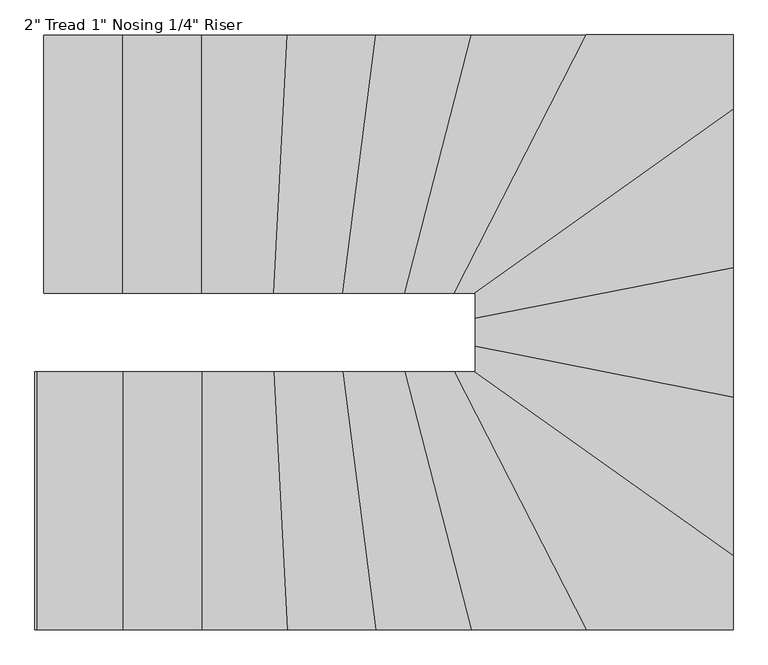
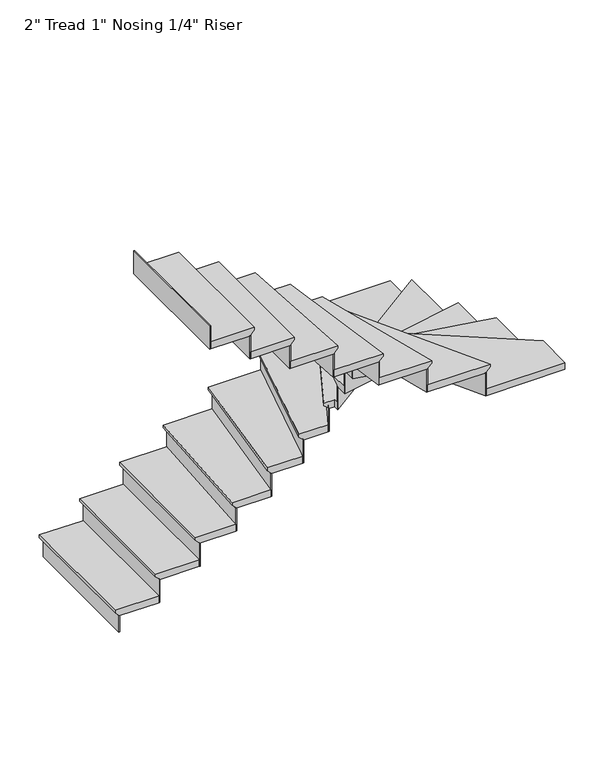
"""IFC4 building model written with IfcOpenShell, lengths in millimetres: stair flight geometry."""

from ifc_helpers import new_model, si_unit, origin, place, context, project, spatial, faceted_brep, source, transform, mapped, element, save


def stair_flight_469f198f(model_context):
    return source(origin(), model_context, "Body", "Brep", [
        faceted_brep([(-3203.9558053, -1112.1366944, 150.2833333), (-3203.9558053, -1112.1366944, 169.3333333), (-3203.9558053, -197.7366944, 169.3333333), (-3203.9558053, -197.7366944, 150.2833333), (-3178.5558053, -1112.1366944, 124.8833333), (-3178.5558053, -197.7366944, 124.8833333), (-2899.1558053, -1112.1366944, 169.3333333), (-2899.1558053, -197.7366944, 169.3333333), (-3178.5558053, -197.7366944, 118.5333333), (-2899.1558053, -197.7366944, 118.5333333), (-2899.1558053, -1112.1366944, 118.5333333), (-3178.5558053, -1112.1366944, 118.5333333)], [[[0, 1, 2, 3]], [[4, 0, 3, 5]], [[2, 1, 6, 7]], [[8, 9, 10, 11]], [[2, 7, 9, 8, 5, 3]], [[8, 11, 4, 5]], [[6, 1, 0, 4, 11, 10]], [[7, 6, 10, 9]]]),
        faceted_brep([(-3178.5558053, -1112.1366944, 118.5333333), (-3178.5558053, -1112.1366944, 0.0), (-3172.2058053, -1112.1366944, 0.0), (-3172.2058053, -1112.1366944, 118.5333333), (-3178.5558053, -197.7366944, 118.5333333), (-3172.2058053, -197.7366944, 118.5333333), (-3172.2058053, -197.7366944, 0.0), (-3178.5558053, -197.7366944, 0.0)], [[[0, 1, 2, 3]], [[4, 5, 6, 7]], [[1, 0, 4, 7]], [[2, 1, 7, 6]], [[3, 2, 6, 5]], [[0, 3, 5, 4]]]),
        faceted_brep([(-2899.1558053, -1112.1366944, 287.8666667), (-2899.1558053, -1112.1366944, 118.5333333), (-2892.8058053, -1112.1366944, 118.5333333), (-2892.8058053, -1112.1366944, 287.8666667), (-2899.1558053, -197.7366944, 287.8666667), (-2892.8058053, -197.7366944, 287.8666667), (-2892.8058053, -197.7366944, 118.5333333), (-2899.1558053, -197.7366944, 118.5333333)], [[[0, 1, 2, 3]], [[4, 5, 6, 7]], [[1, 0, 4, 7]], [[2, 1, 7, 6]], [[3, 2, 6, 5]], [[0, 3, 5, 4]]]),
        faceted_brep([(-2924.5558053, -197.7366944, 338.6666667), (-2924.5558053, -1112.1366944, 338.6666667), (-2619.7558053, -1112.1366944, 338.6666667), (-2619.7558053, -197.7366944, 338.6666667), (-2899.1558053, -197.7366944, 287.8666667), (-2619.7558053, -197.7366944, 287.8666667), (-2619.7558053, -1112.1366944, 287.8666667), (-2899.1558053, -1112.1366944, 287.8666667), (-2899.1558053, -197.7366944, 294.2166667), (-2924.5558053, -197.7366944, 319.6166667), (-2899.1558053, -1112.1366944, 294.2166667), (-2924.5558053, -1112.1366944, 319.6166667)], [[[0, 1, 2, 3]], [[4, 5, 6, 7]], [[0, 3, 5, 4, 8, 9]], [[4, 7, 10, 8]], [[2, 1, 11, 10, 7, 6]], [[3, 2, 6, 5]], [[11, 1, 0, 9]], [[10, 11, 9, 8]]]),
        faceted_brep([(-2619.7558053, -1112.1366944, 457.2), (-2619.7558053, -1112.1366944, 287.8666667), (-2613.4058053, -1112.1366944, 287.8666667), (-2613.4058053, -1112.1366944, 457.2), (-2619.7558053, -197.7366944, 457.2), (-2613.4058053, -197.7366944, 457.2), (-2613.4058053, -197.7366944, 287.8666667), (-2619.7558053, -197.7366944, 287.8666667)], [[[0, 1, 2, 3]], [[4, 5, 6, 7]], [[1, 0, 4, 7]], [[2, 1, 7, 6]], [[3, 2, 6, 5]], [[0, 3, 5, 4]]]),
        faceted_brep([(-2645.1558053, -197.7366944, 508.0), (-2645.1558053, -1112.1366944, 508.0), (-2364.0886438, -1112.1366944, 508.0), (-2316.5543734, -197.7366944, 508.0), (-2619.7558053, -197.7366944, 457.2), (-2316.5543734, -197.7366944, 457.2), (-2364.0886438, -1112.1366944, 457.2), (-2619.7558053, -1112.1366944, 457.2), (-2619.7558053, -197.7366944, 463.55), (-2645.1558053, -197.7366944, 488.95), (-2619.7558053, -1112.1366944, 463.55), (-2645.1558053, -1112.1366944, 488.95)], [[[0, 1, 2, 3]], [[4, 5, 6, 7]], [[0, 3, 5, 4, 8, 9]], [[4, 7, 10, 8]], [[2, 1, 11, 10, 7, 6]], [[3, 2, 6, 5]], [[11, 1, 0, 9]], [[10, 11, 9, 8]]]),
        faceted_brep([(-2364.0886438, -1112.1366944, 626.5333333), (-2364.0886438, -1112.1366944, 457.2), (-2357.7300696, -1112.1366944, 457.2), (-2357.7300696, -1112.1366944, 626.5333333), (-2316.5543734, -197.7366944, 626.5333333), (-2310.1957992, -197.7366944, 626.5333333), (-2310.1957992, -197.7366944, 457.2), (-2316.5543734, -197.7366944, 457.2)], [[[0, 1, 2, 3]], [[4, 5, 6, 7]], [[1, 0, 4, 7]], [[2, 1, 7, 6]], [[3, 2, 6, 5]], [[0, 3, 5, 4]]]),
        faceted_brep([(-2341.9886701, -197.7366944, 677.3333333), (-2389.5229405, -1112.1366944, 677.3333333), (-2119.921944, -1112.1366944, 677.3333333), (-2001.5658923, -197.7366944, 677.3333333), (-2316.5543734, -197.7366944, 626.5333333), (-2001.5658923, -197.7366944, 626.5333333), (-2119.921944, -1112.1366944, 626.5333333), (-2364.0886438, -1112.1366944, 626.5333333), (-2316.5543734, -197.7366944, 632.8833333), (-2341.9886701, -197.7366944, 658.2833333), (-2364.0886438, -1112.1366944, 632.8833333), (-2389.5229405, -1112.1366944, 658.2833333)], [[[0, 1, 2, 3]], [[4, 5, 6, 7]], [[0, 3, 5, 4, 8, 9]], [[4, 7, 10, 8]], [[2, 1, 11, 10, 7, 6]], [[3, 2, 6, 5]], [[11, 1, 0, 9]], [[10, 11, 9, 8]]]),
        faceted_brep([(-2119.921944, -1112.1366944, 795.8666667), (-2119.921944, -1112.1366944, 626.5333333), (-2113.5189722, -1112.1366944, 626.5333333), (-2113.5189722, -1112.1366944, 795.8666667), (-2001.5658923, -197.7366944, 795.8666667), (-1995.1629205, -197.7366944, 795.8666667), (-1995.1629205, -197.7366944, 626.5333333), (-2001.5658923, -197.7366944, 626.5333333)], [[[0, 1, 2, 3]], [[4, 5, 6, 7]], [[1, 0, 4, 7]], [[2, 1, 7, 6]], [[3, 2, 6, 5]], [[0, 3, 5, 4]]]),
        faceted_brep([(-2027.1777794, -197.7366944, 846.6666667), (-2145.5338311, -1112.1366944, 846.6666667), (-1898.2947215, -1112.1366944, 846.6666667), (-1663.1642741, -197.7366944, 846.6666667), (-2001.5658923, -197.7366944, 795.8666667), (-1663.1642741, -197.7366944, 795.8666667), (-1898.2947215, -1112.1366944, 795.8666667), (-2119.921944, -1112.1366944, 795.8666667), (-2001.5658923, -197.7366944, 802.2166667), (-2027.1777794, -197.7366944, 827.6166667), (-2119.921944, -1112.1366944, 802.2166667), (-2145.5338311, -1112.1366944, 827.6166667)], [[[0, 1, 2, 3]], [[4, 5, 6, 7]], [[0, 3, 5, 4, 8, 9]], [[4, 7, 10, 8]], [[2, 1, 11, 10, 7, 6]], [[3, 2, 6, 5]], [[11, 1, 0, 9]], [[10, 11, 9, 8]]]),
        faceted_brep([(-1898.2947215, -1112.1366944, 965.2), (-1898.2947215, -1112.1366944, 795.8666667), (-1891.7381446, -1112.1366944, 795.8666667), (-1891.7381446, -1112.1366944, 965.2), (-1663.1642741, -197.7366944, 965.2), (-1656.6076972, -197.7366944, 965.2), (-1656.6076972, -197.7366944, 795.8666667), (-1663.1642741, -197.7366944, 795.8666667)], [[[0, 1, 2, 3]], [[4, 5, 6, 7]], [[1, 0, 4, 7]], [[2, 1, 7, 6]], [[3, 2, 6, 5]], [[0, 3, 5, 4]]]),
        faceted_brep([(-1689.3905816, -197.7366944, 1016.0), (-1924.521029, -1112.1366944, 1016.0), (-1721.9480854, -1112.1366944, 1016.0), (-1253.1234641, -197.7366944, 1016.0), (-1663.1642741, -197.7366944, 965.2), (-1253.1234641, -197.7366944, 965.2), (-1721.9480854, -1112.1366944, 965.2), (-1898.2947215, -1112.1366944, 965.2), (-1663.1642741, -197.7366944, 971.55), (-1689.3905816, -197.7366944, 996.95), (-1898.2947215, -1112.1366944, 971.55), (-1924.521029, -1112.1366944, 996.95)], [[[0, 1, 2, 3]], [[4, 5, 6, 7]], [[0, 3, 5, 4, 8, 9]], [[4, 7, 10, 8]], [[2, 1, 11, 10, 7, 6]], [[3, 2, 6, 5]], [[11, 1, 0, 9]], [[10, 11, 9, 8]]]),
        faceted_brep([(-1721.9480854, -1112.1366944, 1134.5333333), (-1721.9480854, -1112.1366944, 965.2), (-1714.8121023, -1112.1366944, 965.2), (-1714.8121023, -1112.1366944, 1134.5333333), (-1253.1234641, -197.7366944, 1134.5333333), (-1245.987481, -197.7366944, 1134.5333333), (-1245.987481, -197.7366944, 965.2), (-1253.1234641, -197.7366944, 965.2)], [[[0, 1, 2, 3]], [[4, 5, 6, 7]], [[1, 0, 4, 7]], [[2, 1, 7, 6]], [[3, 2, 6, 5]], [[0, 3, 5, 4]]]),
        faceted_brep([(-761.8241134, -491.4178281, 1185.3333333), (-761.8241134, -197.7366944, 1185.3333333), (-1281.6673966, -197.7366944, 1185.3333333), (-1750.492018, -1112.1366944, 1185.3333333), (-1676.2241134, -1112.1366944, 1185.3333333), (-1676.2241134, -1141.6917772, 1185.3333333), (-761.8241134, -197.7366944, 1134.5333333), (-761.8241134, -491.4178281, 1134.5333333), (-1676.2241134, -1141.6917772, 1134.5333333), (-1676.2241134, -1112.1366944, 1134.5333333), (-1721.9480854, -1112.1366944, 1134.5333333), (-1253.1234641, -197.7366944, 1134.5333333), (-1253.1234641, -197.7366944, 1140.8833333), (-1281.6673966, -197.7366944, 1166.2833333), (-1721.9480854, -1112.1366944, 1140.8833333), (-1750.492018, -1112.1366944, 1166.2833333)], [[[0, 1, 2, 3, 4, 5]], [[6, 7, 8, 9, 10, 11]], [[1, 0, 7, 6]], [[2, 1, 6, 11, 12, 13]], [[11, 10, 14, 12]], [[4, 3, 15, 14, 10, 9]], [[5, 4, 9, 8]], [[0, 5, 8, 7]], [[15, 3, 2, 13]], [[14, 15, 13, 12]]]),
        faceted_brep([(-1676.2241134, -1141.6917772, 1303.8666667), (-1676.2241134, -1141.6917772, 1134.5333333), (-1676.2241134, -1149.483752, 1134.5333333), (-1676.2241134, -1149.483752, 1303.8666667), (-761.8241134, -491.4178281, 1303.8666667), (-761.8241134, -499.2098029, 1303.8666667), (-761.8241134, -499.2098029, 1134.5333333), (-761.8241134, -491.4178281, 1134.5333333)], [[[0, 1, 2, 3]], [[4, 5, 6, 7]], [[1, 0, 4, 7]], [[2, 1, 7, 6]], [[3, 2, 6, 5]], [[0, 3, 5, 4]]]),
        faceted_brep([(-761.8241134, -460.2499289, 1354.6666667), (-1676.2241134, -1110.523878, 1354.6666667), (-1676.2241134, -1228.1458643, 1354.6666667), (-761.8241134, -1047.905008, 1354.6666667), (-761.8241134, -491.4178281, 1303.8666667), (-761.8241134, -1047.905008, 1303.8666667), (-1676.2241134, -1228.1458643, 1303.8666667), (-1676.2241134, -1141.6917772, 1303.8666667), (-761.8241134, -491.4178281, 1310.2166667), (-761.8241134, -460.2499289, 1335.6166667), (-1676.2241134, -1141.6917772, 1310.2166667), (-1676.2241134, -1110.523878, 1335.6166667)], [[[0, 1, 2, 3]], [[4, 5, 6, 7]], [[0, 3, 5, 4, 8, 9]], [[4, 7, 10, 8]], [[2, 1, 11, 10, 7, 6]], [[3, 2, 6, 5]], [[11, 1, 0, 9]], [[10, 11, 9, 8]]]),
        faceted_brep([(-1676.2241134, -1228.1458643, 1473.2), (-1676.2241134, -1228.1458643, 1303.8666667), (-1676.2241134, -1234.6180497, 1303.8666667), (-1676.2241134, -1234.6180497, 1473.2), (-761.8241134, -1047.905008, 1473.2), (-761.8241134, -1054.3771934, 1473.2), (-761.8241134, -1054.3771934, 1303.8666667), (-761.8241134, -1047.905008, 1303.8666667)], [[[0, 1, 2, 3]], [[4, 5, 6, 7]], [[1, 0, 4, 7]], [[2, 1, 7, 6]], [[3, 2, 6, 5]], [[0, 3, 5, 4]]]),
        faceted_brep([(-761.8241134, -1022.0162662, 1524.0), (-1676.2241134, -1202.2571225, 1524.0), (-1676.2241134, -1327.305008, 1524.0), (-761.8241134, -1507.5458643, 1524.0), (-761.8241134, -1047.905008, 1473.2), (-761.8241134, -1507.5458643, 1473.2), (-1676.2241134, -1327.305008, 1473.2), (-1676.2241134, -1228.1458643, 1473.2), (-761.8241134, -1047.905008, 1479.55), (-761.8241134, -1022.0162662, 1504.95), (-1676.2241134, -1228.1458643, 1479.55), (-1676.2241134, -1202.2571225, 1504.95)], [[[0, 1, 2, 3]], [[4, 5, 6, 7]], [[0, 3, 5, 4, 8, 9]], [[4, 7, 10, 8]], [[2, 1, 11, 10, 7, 6]], [[3, 2, 6, 5]], [[11, 1, 0, 9]], [[10, 11, 9, 8]]]),
        faceted_brep([(-1676.2241134, -1327.305008, 1642.5333333), (-1676.2241134, -1327.305008, 1473.2), (-1676.2241134, -1333.7771934, 1473.2), (-1676.2241134, -1333.7771934, 1642.5333333), (-761.8241134, -1507.5458643, 1642.5333333), (-761.8241134, -1514.0180497, 1642.5333333), (-761.8241134, -1514.0180497, 1473.2), (-761.8241134, -1507.5458643, 1473.2)], [[[0, 1, 2, 3]], [[4, 5, 6, 7]], [[1, 0, 4, 7]], [[2, 1, 7, 6]], [[3, 2, 6, 5]], [[0, 3, 5, 4]]]),
        faceted_brep([(-761.8241134, -1481.6571225, 1693.3333333), (-1676.2241134, -1301.4162662, 1693.3333333), (-1676.2241134, -1391.5366944, 1693.3333333), (-1722.3195879, -1391.5366944, 1693.3333333), (-761.8241134, -2074.591359, 1693.3333333), (-761.8241134, -1507.5458643, 1642.5333333), (-761.8241134, -2074.591359, 1642.5333333), (-1722.3195879, -1391.5366944, 1642.5333333), (-1676.2241134, -1391.5366944, 1642.5333333), (-1676.2241134, -1327.305008, 1642.5333333), (-761.8241134, -1507.5458643, 1648.8833333), (-761.8241134, -1481.6571225, 1674.2833333), (-1676.2241134, -1327.305008, 1648.8833333), (-1676.2241134, -1301.4162662, 1674.2833333)], [[[0, 1, 2, 3, 4]], [[5, 6, 7, 8, 9]], [[0, 4, 6, 5, 10, 11]], [[5, 9, 12, 10]], [[2, 1, 13, 12, 9, 8]], [[3, 2, 8, 7]], [[4, 3, 7, 6]], [[13, 1, 0, 11]], [[12, 13, 11, 10]]]),
        faceted_brep([(-1722.3195879, -1391.5366944, 1811.8666667), (-1722.3195879, -1391.5366944, 1642.5333333), (-1733.2764804, -1391.5366944, 1642.5333333), (-1733.2764804, -1391.5366944, 1811.8666667), (-761.8241134, -2074.591359, 1811.8666667), (-761.8241134, -2082.3833338, 1811.8666667), (-761.8241134, -2082.3833338, 1642.5333333), (-761.8241134, -2074.591359, 1642.5333333)], [[[0, 1, 2, 3]], [[4, 5, 6, 7]], [[1, 0, 4, 7]], [[2, 1, 7, 6]], [[3, 2, 6, 5]], [[0, 3, 5, 4]]]),
        faceted_brep([(-1310.2113292, -2305.9366944, 1862.6666667), (-761.8241134, -2305.9366944, 1862.6666667), (-761.8241134, -2043.4234599, 1862.6666667), (-1678.492018, -1391.5366944, 1862.6666667), (-1779.0359505, -1391.5366944, 1862.6666667), (-761.8241134, -2305.9366944, 1811.8666667), (-1310.2113292, -2305.9366944, 1811.8666667), (-1779.0359505, -1391.5366944, 1811.8666667), (-1722.3195879, -1391.5366944, 1811.8666667), (-761.8241134, -2074.591359, 1811.8666667), (-761.8241134, -2074.591359, 1818.2166667), (-761.8241134, -2043.4234599, 1843.6166667), (-1722.3195879, -1391.5366944, 1818.2166667), (-1678.492018, -1391.5366944, 1843.6166667)], [[[0, 1, 2, 3, 4]], [[5, 6, 7, 8, 9]], [[1, 0, 6, 5]], [[2, 1, 5, 9, 10, 11]], [[9, 8, 12, 10]], [[4, 3, 13, 12, 8, 7]], [[0, 4, 7, 6]], [[13, 3, 2, 11]], [[12, 13, 11, 10]]]),
        faceted_brep([(-1779.0359505, -1391.5366944, 1981.2), (-1779.0359505, -1391.5366944, 1811.8666667), (-1786.1719336, -1391.5366944, 1811.8666667), (-1786.1719336, -1391.5366944, 1981.2), (-1310.2113292, -2305.9366944, 1981.2), (-1317.3473123, -2305.9366944, 1981.2), (-1317.3473123, -2305.9366944, 1811.8666667), (-1310.2113292, -2305.9366944, 1811.8666667)], [[[0, 1, 2, 3]], [[4, 5, 6, 7]], [[1, 0, 4, 7]], [[2, 1, 7, 6]], [[3, 2, 6, 5]], [[0, 3, 5, 4]]]),
        faceted_brep([(-1281.6673966, -2305.9366944, 2032.0), (-1750.492018, -1391.5366944, 2032.0), (-1950.7473364, -1391.5366944, 2032.0), (-1715.616889, -2305.9366944, 2032.0), (-1310.2113292, -2305.9366944, 1981.2), (-1715.616889, -2305.9366944, 1981.2), (-1950.7473364, -1391.5366944, 1981.2), (-1779.0359505, -1391.5366944, 1981.2), (-1310.2113292, -2305.9366944, 1987.55), (-1281.6673966, -2305.9366944, 2012.95), (-1779.0359505, -1391.5366944, 1987.55), (-1750.492018, -1391.5366944, 2012.95)], [[[0, 1, 2, 3]], [[4, 5, 6, 7]], [[0, 3, 5, 4, 8, 9]], [[4, 7, 10, 8]], [[2, 1, 11, 10, 7, 6]], [[3, 2, 6, 5]], [[11, 1, 0, 9]], [[10, 11, 9, 8]]]),
        faceted_brep([(-1950.7473364, -1391.5366944, 2150.5333333), (-1950.7473364, -1391.5366944, 1981.2), (-1957.3039133, -1391.5366944, 1981.2), (-1957.3039133, -1391.5366944, 2150.5333333), (-1715.616889, -2305.9366944, 2150.5333333), (-1722.1734659, -2305.9366944, 2150.5333333), (-1722.1734659, -2305.9366944, 1981.2), (-1715.616889, -2305.9366944, 1981.2)], [[[0, 1, 2, 3]], [[4, 5, 6, 7]], [[1, 0, 4, 7]], [[2, 1, 7, 6]], [[3, 2, 6, 5]], [[0, 3, 5, 4]]]),
        faceted_brep([(-1689.3905816, -2305.9366944, 2201.3333333), (-1924.521029, -1391.5366944, 2201.3333333), (-2171.1457182, -1391.5366944, 2201.3333333), (-2052.7896666, -2305.9366944, 2201.3333333), (-1715.616889, -2305.9366944, 2150.5333333), (-2052.7896666, -2305.9366944, 2150.5333333), (-2171.1457182, -1391.5366944, 2150.5333333), (-1950.7473364, -1391.5366944, 2150.5333333), (-1715.616889, -2305.9366944, 2156.8833333), (-1689.3905816, -2305.9366944, 2182.2833333), (-1950.7473364, -1391.5366944, 2156.8833333), (-1924.521029, -1391.5366944, 2182.2833333)], [[[0, 1, 2, 3]], [[4, 5, 6, 7]], [[0, 3, 5, 4, 8, 9]], [[4, 7, 10, 8]], [[2, 1, 11, 10, 7, 6]], [[3, 2, 6, 5]], [[11, 1, 0, 9]], [[10, 11, 9, 8]]]),
        faceted_brep([(-2171.1457182, -1391.5366944, 2319.8666667), (-2171.1457182, -1391.5366944, 2150.5333333), (-2177.54869, -1391.5366944, 2150.5333333), (-2177.54869, -1391.5366944, 2319.8666667), (-2052.7896666, -2305.9366944, 2319.8666667), (-2059.1926383, -2305.9366944, 2319.8666667), (-2059.1926383, -2305.9366944, 2150.5333333), (-2052.7896666, -2305.9366944, 2150.5333333)], [[[0, 1, 2, 3]], [[4, 5, 6, 7]], [[1, 0, 4, 7]], [[2, 1, 7, 6]], [[3, 2, 6, 5]], [[0, 3, 5, 4]]]),
        faceted_brep([(-2027.1777794, -2305.9366944, 2370.6666667), (-2145.5338311, -1391.5366944, 2370.6666667), (-2414.9572371, -1391.5366944, 2370.6666667), (-2367.4229667, -2305.9366944, 2370.6666667), (-2052.7896666, -2305.9366944, 2319.8666667), (-2367.4229667, -2305.9366944, 2319.8666667), (-2414.9572371, -1391.5366944, 2319.8666667), (-2171.1457182, -1391.5366944, 2319.8666667), (-2052.7896666, -2305.9366944, 2326.2166667), (-2027.1777794, -2305.9366944, 2351.6166667), (-2171.1457182, -1391.5366944, 2326.2166667), (-2145.5338311, -1391.5366944, 2351.6166667)], [[[0, 1, 2, 3]], [[4, 5, 6, 7]], [[0, 3, 5, 4, 8, 9]], [[4, 7, 10, 8]], [[2, 1, 11, 10, 7, 6]], [[3, 2, 6, 5]], [[11, 1, 0, 9]], [[10, 11, 9, 8]]]),
        faceted_brep([(-2414.9572371, -1391.5366944, 2489.2), (-2414.9572371, -1391.5366944, 2319.8666667), (-2421.3158113, -1391.5366944, 2319.8666667), (-2421.3158113, -1391.5366944, 2489.2), (-2367.4229667, -2305.9366944, 2489.2), (-2373.7815409, -2305.9366944, 2489.2), (-2373.7815409, -2305.9366944, 2319.8666667), (-2367.4229667, -2305.9366944, 2319.8666667)], [[[0, 1, 2, 3]], [[4, 5, 6, 7]], [[1, 0, 4, 7]], [[2, 1, 7, 6]], [[3, 2, 6, 5]], [[0, 3, 5, 4]]]),
        faceted_brep([(-2341.9886701, -2305.9366944, 2540.0), (-2389.5229405, -1391.5366944, 2540.0), (-2670.5558053, -1391.5366944, 2540.0), (-2670.5558053, -2305.9366944, 2540.0), (-2367.4229667, -2305.9366944, 2489.2), (-2670.5558053, -2305.9366944, 2489.2), (-2670.5558053, -1391.5366944, 2489.2), (-2414.9572371, -1391.5366944, 2489.2), (-2367.4229667, -2305.9366944, 2495.55), (-2341.9886701, -2305.9366944, 2520.95), (-2414.9572371, -1391.5366944, 2495.55), (-2389.5229405, -1391.5366944, 2520.95)], [[[0, 1, 2, 3]], [[4, 5, 6, 7]], [[0, 3, 5, 4, 8, 9]], [[4, 7, 10, 8]], [[2, 1, 11, 10, 7, 6]], [[3, 2, 6, 5]], [[11, 1, 0, 9]], [[10, 11, 9, 8]]]),
        faceted_brep([(-2670.5558053, -1391.5366944, 2658.5333333), (-2670.5558053, -1391.5366944, 2489.2), (-2676.9058053, -1391.5366944, 2489.2), (-2676.9058053, -1391.5366944, 2658.5333333), (-2670.5558053, -2305.9366944, 2658.5333333), (-2676.9058053, -2305.9366944, 2658.5333333), (-2676.9058053, -2305.9366944, 2489.2), (-2670.5558053, -2305.9366944, 2489.2)], [[[0, 1, 2, 3]], [[4, 5, 6, 7]], [[1, 0, 4, 7]], [[2, 1, 7, 6]], [[3, 2, 6, 5]], [[0, 3, 5, 4]]]),
        faceted_brep([(-2645.1558053, -2305.9366944, 2709.3333333), (-2645.1558053, -1391.5366944, 2709.3333333), (-2949.9558053, -1391.5366944, 2709.3333333), (-2949.9558053, -2305.9366944, 2709.3333333), (-2670.5558053, -2305.9366944, 2658.5333333), (-2949.9558053, -2305.9366944, 2658.5333333), (-2949.9558053, -1391.5366944, 2658.5333333), (-2670.5558053, -1391.5366944, 2658.5333333), (-2670.5558053, -2305.9366944, 2664.8833333), (-2645.1558053, -2305.9366944, 2690.2833333), (-2670.5558053, -1391.5366944, 2664.8833333), (-2645.1558053, -1391.5366944, 2690.2833333)], [[[0, 1, 2, 3]], [[4, 5, 6, 7]], [[0, 3, 5, 4, 8, 9]], [[4, 7, 10, 8]], [[2, 1, 11, 10, 7, 6]], [[3, 2, 6, 5]], [[11, 1, 0, 9]], [[10, 11, 9, 8]]]),
        faceted_brep([(-2949.9558053, -1391.5366944, 2827.8666667), (-2949.9558053, -1391.5366944, 2658.5333333), (-2956.3058053, -1391.5366944, 2658.5333333), (-2956.3058053, -1391.5366944, 2827.8666667), (-2949.9558053, -2305.9366944, 2827.8666667), (-2956.3058053, -2305.9366944, 2827.8666667), (-2956.3058053, -2305.9366944, 2658.5333333), (-2949.9558053, -2305.9366944, 2658.5333333)], [[[0, 1, 2, 3]], [[4, 5, 6, 7]], [[1, 0, 4, 7]], [[2, 1, 7, 6]], [[3, 2, 6, 5]], [[0, 3, 5, 4]]]),
        faceted_brep([(-3229.3558053, -1391.5366944, 2997.2), (-3229.3558053, -1391.5366944, 2827.8666667), (-3235.7058053, -1391.5366944, 2827.8666667), (-3235.7058053, -1391.5366944, 2997.2), (-3229.3558053, -2305.9366944, 2997.2), (-3235.7058053, -2305.9366944, 2997.2), (-3235.7058053, -2305.9366944, 2827.8666667), (-3229.3558053, -2305.9366944, 2827.8666667)], [[[0, 1, 2, 3]], [[4, 5, 6, 7]], [[1, 0, 4, 7]], [[2, 1, 7, 6]], [[3, 2, 6, 5]], [[0, 3, 5, 4]]]),
        faceted_brep([(-2924.5558053, -2305.9366944, 2878.6666667), (-2924.5558053, -1391.5366944, 2878.6666667), (-3229.3558053, -1391.5366944, 2878.6666667), (-3229.3558053, -2305.9366944, 2878.6666667), (-2949.9558053, -2305.9366944, 2827.8666667), (-3229.3558053, -2305.9366944, 2827.8666667), (-3229.3558053, -1391.5366944, 2827.8666667), (-2949.9558053, -1391.5366944, 2827.8666667), (-2949.9558053, -2305.9366944, 2834.2166667), (-2924.5558053, -2305.9366944, 2859.6166667), (-2949.9558053, -1391.5366944, 2834.2166667), (-2924.5558053, -1391.5366944, 2859.6166667)], [[[0, 1, 2, 3]], [[4, 5, 6, 7]], [[0, 3, 5, 4, 8, 9]], [[4, 7, 10, 8]], [[2, 1, 11, 10, 7, 6]], [[3, 2, 6, 5]], [[11, 1, 0, 9]], [[10, 11, 9, 8]]]),
    ])


if __name__ == "__main__":
    model = new_model("IFC4")
    model_context = context("Model", 3, world=origin())
    ifc_project = project(units=[si_unit("LENGTHUNIT", "METRE", prefix="MILLI")], contexts=[model_context])
    site = spatial("IfcSite", under=ifc_project)
    building = spatial("IfcBuilding", under=site)
    placement = place(None, origin())
    stair_flight_shape = stair_flight_469f198f(model_context)
    element("IfcStairFlight", 1, ObjectType="2\" Tread 1\" Nosing 1/4\" Riser", at=placement, inside=building, context=model_context, shape_type="MappedRepresentation", body=[
        mapped(stair_flight_shape, transform((0.0, 0.0, 0.0), x_axis=(1.0, 0.0, 0.0), y_axis=(0.0, 1.0, 0.0), z_axis=(0.0, 0.0, 1.0))),
    ])
    save(model, "model.ifc")
